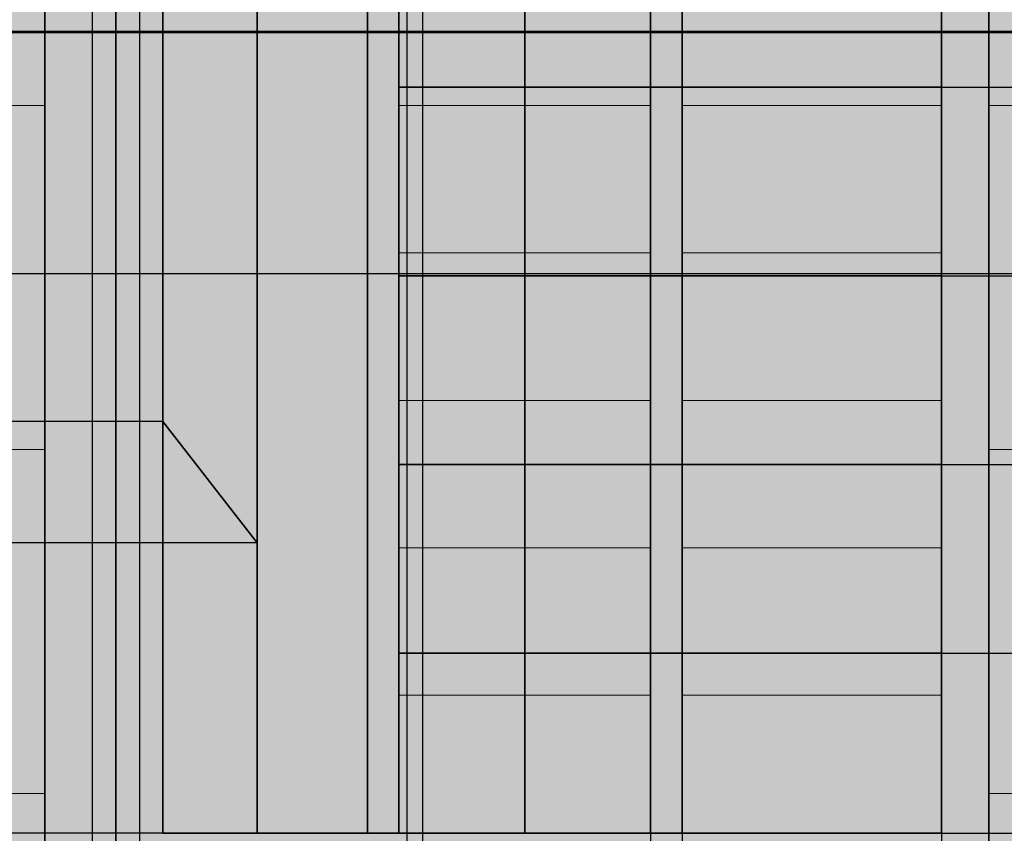
# Model space of a CAD drawing. Units: inches. Extents: x 148 to 1080, y 89 to 707.
# Tile 3 of 12: x 272 to 397, y 170 to 273. Entities that reach past the tile are written whole.
import ezdxf

# ---------------------------------------------------------------- set-up
doc = ezdxf.new("R2010")
doc.units = ezdxf.units.IN
doc.header["$MEASUREMENT"] = 0
for name, color, linetype, lineweight in [('A-ANNO-DIMS', 2, 'Continuous', 18), ('A-ELEV', 7, 'Continuous', 35), ('A-ELEV-PATT', 8, 'Continuous', 13)]:
    doc.layers.add(name, color=color, linetype=linetype, lineweight=lineweight)
doc.styles.get("Standard").update_dxf_attribs({"font": 'arial.ttf'})
doc.dimstyles.get("Standard").update_dxf_attribs({"dimtxt": 6, "dimasz": 0.18, "dimexe": 0.18, "dimexo": 0.0625, "dimgap": 0.09, "dimtad": 0, "dimtih": 1, "dimtoh": 1, "dimdec": 0, "dimzin": 0, "dimdsep": 46, "dimlunit": 3, "dimtxsty": 'Standard', "dimcen": 0.09, "dimadec": 0, "dimazin": 0, "dimtfac": 1, "dimtdec": 0, "dimtofl": 0, "dimtmove": 0, "dimatfit": 3, "dimfxl": 1, "dimtolj": 1, "dimtzin": 0, "dimarcsym": 0})

# ---------------------------------------------------------------- blocks, each defined once
blk = doc.blocks.new('*D28')
at = {"layer": 'A-ANNO-DIMS', "color": 0, "lineweight": -2, "transparency": 16777216}
for p, q in [((274.96, 331.95), (160.42, 331.95)), ((160.6, 331.77), (160.6, 251.1)), ((160.6, 164.13), (160.6, 244.79)), ((274.96, 163.95), (160.42, 163.95))]:
    blk.add_line(p, q, dxfattribs=at)
at = {"layer": 'A-ANNO-DIMS', "color": 0, "transparency": 16777216}
for points in [[(160.57, 331.77), (160.63, 331.77), (160.6, 331.95)], [(160.57, 164.13), (160.63, 164.13), (160.6, 163.95)]]:
    blk.add_solid(points, dxfattribs=at)
at = {"layer": 'Defpoints', "color": 0, "transparency": 16777216}
for p in [(160.6, 331.95), (275.02, 331.95), (275.02, 163.95)]:
    blk.add_point(p, dxfattribs=at)
at = {"layer": 'A-ANNO-DIMS', "color": 0, "transparency": 16777216, "insert": (160.6, 247.95), "char_height": 6, "attachment_point": 5}
blk.add_mtext('\\A1;168', dxfattribs=at)
blk = doc.blocks.new('*D32')
at = {"layer": 'A-ANNO-DIMS', "color": 0, "lineweight": -2, "transparency": 16777216}
for p, q in [((587, 271.77), (160.42, 271.77)), ((160.6, 271.59), (160.6, 213.18)), ((160.6, 148.46), (160.6, 206.87)), ((587, 148.28), (160.42, 148.28))]:
    blk.add_line(p, q, dxfattribs=at)
at = {"layer": 'A-ANNO-DIMS', "color": 0, "transparency": 16777216}
for points in [[(160.57, 271.59), (160.63, 271.59), (160.6, 271.77)], [(160.57, 148.46), (160.63, 148.46), (160.6, 148.28)]]:
    blk.add_solid(points, dxfattribs=at)
at = {"layer": 'Defpoints', "color": 0, "transparency": 16777216}
for p in [(160.6, 271.77), (587.06, 271.77), (587.06, 148.28)]:
    blk.add_point(p, dxfattribs=at)
at = {"layer": 'A-ANNO-DIMS', "color": 0, "transparency": 16777216, "insert": (160.6, 210.03), "char_height": 6, "attachment_point": 5}
blk.add_mtext('\\A1;123.5', dxfattribs=at)
blk = doc.blocks.new('*D34')
at = {"layer": 'A-ANNO-DIMS', "color": 0, "lineweight": -2, "transparency": 16777216}
for p, q in [((574.96, 283.95), (160.42, 283.95)), ((160.6, 283.77), (160.6, 212.1)), ((160.6, 134.13), (160.6, 205.79)), ((574.96, 133.95), (160.42, 133.95))]:
    blk.add_line(p, q, dxfattribs=at)
at = {"layer": 'A-ANNO-DIMS', "color": 0, "transparency": 16777216}
for points in [[(160.57, 283.77), (160.63, 283.77), (160.6, 283.95)], [(160.57, 134.13), (160.63, 134.13), (160.6, 133.95)]]:
    blk.add_solid(points, dxfattribs=at)
at = {"layer": 'Defpoints', "color": 0, "transparency": 16777216}
for p in [(575.02, 283.95), (160.6, 133.95), (575.02, 133.95)]:
    blk.add_point(p, dxfattribs=at)
at = {"layer": 'A-ANNO-DIMS', "color": 0, "transparency": 16777216, "insert": (160.6, 208.95), "char_height": 6, "attachment_point": 5}
blk.add_mtext('\\A1;150', dxfattribs=at)
blk = doc.blocks.new('*D38')
at = {"layer": 'A-ANNO-DIMS', "color": 0, "lineweight": -2, "transparency": 16777216}
for p, q in [((934.89, 271.95), (160.42, 271.95)), ((160.6, 271.77), (160.6, 206.1)), ((160.6, 134.13), (160.6, 199.79)), ((934.89, 133.95), (160.42, 133.95))]:
    blk.add_line(p, q, dxfattribs=at)
at = {"layer": 'A-ANNO-DIMS', "color": 0, "transparency": 16777216}
for points in [[(160.57, 271.77), (160.63, 271.77), (160.6, 271.95)], [(160.57, 134.13), (160.63, 134.13), (160.6, 133.95)]]:
    blk.add_solid(points, dxfattribs=at)
at = {"layer": 'Defpoints', "color": 0, "transparency": 16777216}
for p in [(934.95, 271.95), (160.6, 133.95), (934.95, 133.95)]:
    blk.add_point(p, dxfattribs=at)
at = {"layer": 'A-ANNO-DIMS', "color": 0, "transparency": 16777216, "insert": (160.6, 202.95), "char_height": 6, "attachment_point": 5}
blk.add_mtext('\\A1;138', dxfattribs=at)
blk = doc.blocks.new('*D43')
at = {"layer": 'A-ANNO-DIMS', "color": 0, "lineweight": -2, "transparency": 16777216}
for p, q in [((765.88, 241.1), (160.42, 241.1)), ((160.6, 240.92), (160.6, 190.68)), ((160.6, 134.13), (160.6, 184.37)), ((776.65, 133.95), (160.42, 133.95))]:
    blk.add_line(p, q, dxfattribs=at)
at = {"layer": 'A-ANNO-DIMS', "color": 0, "transparency": 16777216}
for points in [[(160.57, 240.92), (160.63, 240.92), (160.6, 241.1)], [(160.57, 134.13), (160.63, 134.13), (160.6, 133.95)]]:
    blk.add_solid(points, dxfattribs=at)
at = {"layer": 'Defpoints', "color": 0, "transparency": 16777216}
for p in [(765.95, 241.1), (160.6, 133.95), (776.71, 133.95)]:
    blk.add_point(p, dxfattribs=at)
at = {"layer": 'A-ANNO-DIMS', "color": 0, "transparency": 16777216, "insert": (160.6, 187.52), "char_height": 6, "attachment_point": 5}
blk.add_mtext('\\A1;107.15', dxfattribs=at)
blk = doc.blocks.new('*D71')
at = {"layer": 'A-ANNO-DIMS', "color": 0, "lineweight": -2, "transparency": 16777216}
for p, q in [((389.08, 169.95), (1064.5, 169.95)), ((1064.32, 169.95), (1064.32, 170.13)), ((1064.32, 170.13), (1064.5, 170.13)), ((1064.32, 164.13), (1064.32, 169.77)), ((395.08, 163.95), (1064.5, 163.95))]:
    blk.add_line(p, q, dxfattribs=at)
at = {"layer": 'A-ANNO-DIMS', "color": 0, "transparency": 16777216}
for points in [[(1064.29, 169.77), (1064.35, 169.77), (1064.32, 169.95)], [(1064.29, 164.13), (1064.35, 164.13), (1064.32, 163.95)]]:
    blk.add_solid(points, dxfattribs=at)
at = {"layer": 'Defpoints', "color": 0, "transparency": 16777216}
for p in [(389.02, 169.95), (1064.32, 169.95), (395.02, 163.95)]:
    blk.add_point(p, dxfattribs=at)
at = {"layer": 'A-ANNO-DIMS', "color": 0, "transparency": 16777216, "insert": (1072.39, 170.13), "char_height": 6, "attachment_point": 5}
blk.add_mtext('\\A1;6.00', dxfattribs=at)
blk = doc.blocks.new('*D72')
at = {"layer": 'A-ANNO-DIMS', "color": 0, "lineweight": -2, "transparency": 16777216}
for p, q in [((389.08, 192.87), (1064.5, 192.87)), ((1064.32, 192.69), (1064.32, 184.56)), ((1064.32, 170.13), (1064.32, 178.26)), ((389.08, 169.95), (1064.5, 169.95))]:
    blk.add_line(p, q, dxfattribs=at)
at = {"layer": 'A-ANNO-DIMS', "color": 0, "transparency": 16777216}
for points in [[(1064.29, 192.69), (1064.35, 192.69), (1064.32, 192.87)], [(1064.29, 170.13), (1064.35, 170.13), (1064.32, 169.95)]]:
    blk.add_solid(points, dxfattribs=at)
at = {"layer": 'Defpoints', "color": 0, "transparency": 16777216}
for p in [(389.02, 192.87), (1064.32, 192.87), (389.02, 169.95)]:
    blk.add_point(p, dxfattribs=at)
at = {"layer": 'A-ANNO-DIMS', "color": 0, "transparency": 16777216, "insert": (1064.32, 181.41), "char_height": 6, "attachment_point": 5}
blk.add_mtext('\\A1;22.92', dxfattribs=at)
blk = doc.blocks.new('*D73')
at = {"layer": 'A-ANNO-DIMS', "color": 0, "lineweight": -2, "transparency": 16777216}
for p, q in [((389.08, 216.87), (1064.5, 216.87)), ((1064.32, 216.69), (1064.32, 208.02)), ((1064.32, 193.05), (1064.32, 201.72)), ((389.08, 192.87), (1064.5, 192.87))]:
    blk.add_line(p, q, dxfattribs=at)
at = {"layer": 'A-ANNO-DIMS', "color": 0, "transparency": 16777216}
for points in [[(1064.29, 216.69), (1064.35, 216.69), (1064.32, 216.87)], [(1064.29, 193.05), (1064.35, 193.05), (1064.32, 192.87)]]:
    blk.add_solid(points, dxfattribs=at)
at = {"layer": 'Defpoints', "color": 0, "transparency": 16777216}
for p in [(389.02, 216.87), (1064.32, 216.87), (389.02, 192.87)]:
    blk.add_point(p, dxfattribs=at)
at = {"layer": 'A-ANNO-DIMS', "color": 0, "transparency": 16777216, "insert": (1064.32, 204.87), "char_height": 6, "attachment_point": 5}
blk.add_mtext('\\A1;24.00', dxfattribs=at)
blk = doc.blocks.new('*D74')
at = {"layer": 'A-ANNO-DIMS', "color": 0, "lineweight": -2, "transparency": 16777216}
for p, q in [((389.08, 240.87), (1064.5, 240.87)), ((1064.32, 240.69), (1064.32, 232.02)), ((1064.32, 217.05), (1064.32, 225.72)), ((389.08, 216.87), (1064.5, 216.87))]:
    blk.add_line(p, q, dxfattribs=at)
at = {"layer": 'A-ANNO-DIMS', "color": 0, "transparency": 16777216}
for points in [[(1064.29, 240.69), (1064.35, 240.69), (1064.32, 240.87)], [(1064.29, 217.05), (1064.35, 217.05), (1064.32, 216.87)]]:
    blk.add_solid(points, dxfattribs=at)
at = {"layer": 'Defpoints', "color": 0, "transparency": 16777216}
for p in [(389.02, 240.87), (1064.32, 240.87), (389.02, 216.87)]:
    blk.add_point(p, dxfattribs=at)
at = {"layer": 'A-ANNO-DIMS', "color": 0, "transparency": 16777216, "insert": (1064.32, 228.87), "char_height": 6, "attachment_point": 5}
blk.add_mtext('\\A1;24.00', dxfattribs=at)
blk = doc.blocks.new('*D75')
at = {"layer": 'A-ANNO-DIMS', "color": 0, "lineweight": -2, "transparency": 16777216}
for p, q in [((389.08, 264.87), (1064.5, 264.87)), ((1064.32, 264.69), (1064.32, 256.02)), ((1064.32, 241.05), (1064.32, 249.72)), ((389.08, 240.87), (1064.5, 240.87))]:
    blk.add_line(p, q, dxfattribs=at)
at = {"layer": 'A-ANNO-DIMS', "color": 0, "transparency": 16777216}
for points in [[(1064.29, 264.69), (1064.35, 264.69), (1064.32, 264.87)], [(1064.29, 241.05), (1064.35, 241.05), (1064.32, 240.87)]]:
    blk.add_solid(points, dxfattribs=at)
at = {"layer": 'Defpoints', "color": 0, "transparency": 16777216}
for p in [(389.02, 264.87), (1064.32, 264.87), (389.02, 240.87)]:
    blk.add_point(p, dxfattribs=at)
at = {"layer": 'A-ANNO-DIMS', "color": 0, "transparency": 16777216, "insert": (1064.32, 252.87), "char_height": 6, "attachment_point": 5}
blk.add_mtext('\\A1;24.00', dxfattribs=at)
blk = doc.blocks.new('*D76')
at = {"layer": 'A-ANNO-DIMS', "color": 0, "lineweight": -2, "transparency": 16777216}
for p, q in [((389.08, 300.95), (1064.5, 300.95)), ((1064.32, 300.77), (1064.32, 286.06)), ((1064.32, 265.05), (1064.32, 279.75)), ((389.08, 264.87), (1064.5, 264.87))]:
    blk.add_line(p, q, dxfattribs=at)
at = {"layer": 'A-ANNO-DIMS', "color": 0, "transparency": 16777216}
for points in [[(1064.29, 300.77), (1064.35, 300.77), (1064.32, 300.95)], [(1064.29, 265.05), (1064.35, 265.05), (1064.32, 264.87)]]:
    blk.add_solid(points, dxfattribs=at)
at = {"layer": 'Defpoints', "color": 0, "transparency": 16777216}
for p in [(389.02, 300.95), (1064.32, 300.95), (389.02, 264.87)]:
    blk.add_point(p, dxfattribs=at)
at = {"layer": 'A-ANNO-DIMS', "color": 0, "transparency": 16777216, "insert": (1064.32, 282.91), "char_height": 6, "attachment_point": 5}
blk.add_mtext('\\A1;36.08', dxfattribs=at)
blk = doc.blocks.new('*D80')
at = {"layer": 'A-ANNO-DIMS', "color": 0, "lineweight": -2, "transparency": 16777216}
for p, q in [((289.96, 222.32), (160.42, 222.32)), ((160.6, 222.14), (160.6, 199.29)), ((160.6, 170.13), (160.6, 192.98)), ((289.96, 169.95), (160.42, 169.95))]:
    blk.add_line(p, q, dxfattribs=at)
at = {"layer": 'A-ANNO-DIMS', "color": 0, "transparency": 16777216}
for points in [[(160.57, 222.14), (160.63, 222.14), (160.6, 222.32)], [(160.57, 170.13), (160.63, 170.13), (160.6, 169.95)]]:
    blk.add_solid(points, dxfattribs=at)
at = {"layer": 'Defpoints', "color": 0, "transparency": 16777216}
for p in [(160.6, 222.32), (290.02, 222.32), (290.02, 169.95)]:
    blk.add_point(p, dxfattribs=at)
at = {"layer": 'A-ANNO-DIMS', "color": 0, "transparency": 16777216, "insert": (160.6, 196.13), "char_height": 6, "attachment_point": 5}
blk.add_mtext('\\A1;52.37', dxfattribs=at)
blk = doc.blocks.new('*D81')
at = {"layer": 'A-ANNO-DIMS', "color": 0, "lineweight": -2, "transparency": 16777216}
for p, q in [((301.96, 206.89), (160.42, 206.89)), ((160.6, 206.71), (160.6, 191.57)), ((160.6, 170.13), (160.6, 185.26)), ((301.96, 169.95), (160.42, 169.95))]:
    blk.add_line(p, q, dxfattribs=at)
at = {"layer": 'A-ANNO-DIMS', "color": 0, "transparency": 16777216}
for points in [[(160.57, 206.71), (160.63, 206.71), (160.6, 206.89)], [(160.57, 170.13), (160.63, 170.13), (160.6, 169.95)]]:
    blk.add_solid(points, dxfattribs=at)
at = {"layer": 'Defpoints', "color": 0, "transparency": 16777216}
for p in [(160.6, 206.89), (302.02, 206.89), (302.02, 169.95)]:
    blk.add_point(p, dxfattribs=at)
at = {"layer": 'A-ANNO-DIMS', "color": 0, "transparency": 16777216, "insert": (160.6, 188.42), "char_height": 6, "attachment_point": 5}
blk.add_mtext('\\A1;36.944', dxfattribs=at)
blk = doc.blocks.new('*D82')
at = {"layer": 'A-ANNO-DIMS', "color": 0, "lineweight": -2, "transparency": 16777216}
for p, q in [((275.02, 400.88), (275.02, 92.62)), ((281.02, 400.88), (281.02, 92.62)), ((275.2, 92.8), (280.84, 92.8)), ((281.02, 92.8), (281.2, 92.8))]:
    blk.add_line(p, q, dxfattribs=at)
at = {"layer": 'A-ANNO-DIMS', "color": 0, "transparency": 16777216}
for points in [[(275.2, 92.83), (275.2, 92.77), (275.02, 92.8)], [(280.84, 92.83), (280.84, 92.77), (281.02, 92.8)]]:
    blk.add_solid(points, dxfattribs=at)
at = {"layer": 'Defpoints', "color": 0, "transparency": 16777216}
for p in [(275.02, 400.95), (281.02, 400.95), (281.02, 92.8)]:
    blk.add_point(p, dxfattribs=at)
at = {"layer": 'A-ANNO-DIMS', "color": 0, "transparency": 16777216, "insert": (289.09, 92.8), "char_height": 6, "attachment_point": 5}
blk.add_mtext('\\A1;6.00', dxfattribs=at)
blk = doc.blocks.new('*D83')
at = {"layer": 'A-ANNO-DIMS', "color": 0, "lineweight": -2, "transparency": 16777216}
for p, q in [((281.02, 400.88), (281.02, 92.62)), ((287.02, 400.88), (287.02, 92.62)), ((281.2, 92.8), (286.84, 92.8)), ((287.02, 92.8), (287.2, 92.8))]:
    blk.add_line(p, q, dxfattribs=at)
at = {"layer": 'A-ANNO-DIMS', "color": 0, "transparency": 16777216}
for points in [[(281.2, 92.83), (281.2, 92.77), (281.02, 92.8)], [(286.84, 92.83), (286.84, 92.77), (287.02, 92.8)]]:
    blk.add_solid(points, dxfattribs=at)
at = {"layer": 'Defpoints', "color": 0, "transparency": 16777216}
for p in [(281.02, 400.95), (287.02, 400.95), (287.02, 92.8)]:
    blk.add_point(p, dxfattribs=at)
at = {"layer": 'A-ANNO-DIMS', "color": 0, "transparency": 16777216, "insert": (295.09, 92.8), "char_height": 6, "attachment_point": 5}
blk.add_mtext('\\A1;6.00', dxfattribs=at)
blk = doc.blocks.new('*D84')
at = {"layer": 'A-ANNO-DIMS', "color": 0, "lineweight": -2, "transparency": 16777216}
for p, q in [((321.02, 529.88), (321.02, 92.62)), ((287.02, 400.88), (287.02, 92.62)), ((287.2, 92.8), (293.82, 92.8)), ((320.84, 92.8), (314.22, 92.8))]:
    blk.add_line(p, q, dxfattribs=at)
at = {"layer": 'A-ANNO-DIMS', "color": 0, "transparency": 16777216}
for points in [[(287.2, 92.83), (287.2, 92.77), (287.02, 92.8)], [(320.84, 92.83), (320.84, 92.77), (321.02, 92.8)]]:
    blk.add_solid(points, dxfattribs=at)
at = {"layer": 'Defpoints', "color": 0, "transparency": 16777216}
for p in [(321.02, 529.95), (287.02, 400.95), (321.02, 92.8)]:
    blk.add_point(p, dxfattribs=at)
at = {"layer": 'A-ANNO-DIMS', "color": 0, "transparency": 16777216, "insert": (304.02, 92.8), "char_height": 6, "attachment_point": 5}
blk.add_mtext('\\A1;34.00', dxfattribs=at)
blk = doc.blocks.new('*D85')
at = {"layer": 'A-ANNO-DIMS', "color": 0, "lineweight": -2, "transparency": 16777216}
for p, q in [((321.02, 529.88), (321.02, 92.62)), ((323.02, 400.88), (323.02, 92.62)), ((321.2, 92.8), (322.84, 92.8)), ((323.02, 92.8), (323.2, 92.8))]:
    blk.add_line(p, q, dxfattribs=at)
at = {"layer": 'A-ANNO-DIMS', "color": 0, "transparency": 16777216}
for points in [[(321.2, 92.83), (321.2, 92.77), (321.02, 92.8)], [(322.84, 92.83), (322.84, 92.77), (323.02, 92.8)]]:
    blk.add_solid(points, dxfattribs=at)
at = {"layer": 'Defpoints', "color": 0, "transparency": 16777216}
for p in [(321.02, 529.95), (323.02, 400.95), (323.02, 92.8)]:
    blk.add_point(p, dxfattribs=at)
at = {"layer": 'A-ANNO-DIMS', "color": 0, "transparency": 16777216, "insert": (331.12, 92.8), "char_height": 6, "attachment_point": 5}
blk.add_mtext('\\A1;2.00', dxfattribs=at)
blk = doc.blocks.new('*D86')
at = {"layer": 'A-ANNO-DIMS', "color": 0, "lineweight": -2, "transparency": 16777216}
for p, q in [((323.02, 400.88), (323.02, 92.62)), ((352.02, 400.88), (352.02, 92.62)), ((323.2, 92.8), (327.27, 92.8)), ((351.84, 92.8), (347.77, 92.8))]:
    blk.add_line(p, q, dxfattribs=at)
at = {"layer": 'A-ANNO-DIMS', "color": 0, "transparency": 16777216}
for points in [[(323.2, 92.83), (323.2, 92.77), (323.02, 92.8)], [(351.84, 92.83), (351.84, 92.77), (352.02, 92.8)]]:
    blk.add_solid(points, dxfattribs=at)
at = {"layer": 'Defpoints', "color": 0, "transparency": 16777216}
for p in [(323.02, 400.95), (352.02, 400.95), (352.02, 92.8)]:
    blk.add_point(p, dxfattribs=at)
at = {"layer": 'A-ANNO-DIMS', "color": 0, "transparency": 16777216, "insert": (337.52, 92.8), "char_height": 6, "attachment_point": 5}
blk.add_mtext('\\A1;29.00', dxfattribs=at)
blk = doc.blocks.new('*D87')
at = {"layer": 'A-ANNO-DIMS', "color": 0, "lineweight": -2, "transparency": 16777216}
for p, q in [((352.02, 400.88), (352.02, 92.62)), ((356.02, 400.88), (356.02, 92.62)), ((352.2, 92.8), (355.84, 92.8)), ((356.02, 92.8), (356.2, 92.8))]:
    blk.add_line(p, q, dxfattribs=at)
at = {"layer": 'A-ANNO-DIMS', "color": 0, "transparency": 16777216}
for points in [[(352.2, 92.83), (352.2, 92.77), (352.02, 92.8)], [(355.84, 92.83), (355.84, 92.77), (356.02, 92.8)]]:
    blk.add_solid(points, dxfattribs=at)
at = {"layer": 'Defpoints', "color": 0, "transparency": 16777216}
for p in [(352.02, 400.95), (356.02, 400.95), (356.02, 92.8)]:
    blk.add_point(p, dxfattribs=at)
at = {"layer": 'A-ANNO-DIMS', "color": 0, "transparency": 16777216, "insert": (364.19, 92.8), "char_height": 6, "attachment_point": 5}
blk.add_mtext('\\A1;4.00', dxfattribs=at)
blk = doc.blocks.new('*D88')
at = {"layer": 'A-ANNO-DIMS', "color": 0, "lineweight": -2, "transparency": 16777216}
for p, q in [((356.02, 400.88), (356.02, 92.62)), ((389.02, 400.88), (389.02, 92.62)), ((356.2, 92.8), (362.32, 92.8)), ((388.84, 92.8), (382.72, 92.8))]:
    blk.add_line(p, q, dxfattribs=at)
at = {"layer": 'A-ANNO-DIMS', "color": 0, "transparency": 16777216}
for points in [[(356.2, 92.83), (356.2, 92.77), (356.02, 92.8)], [(388.84, 92.83), (388.84, 92.77), (389.02, 92.8)]]:
    blk.add_solid(points, dxfattribs=at)
at = {"layer": 'Defpoints', "color": 0, "transparency": 16777216}
for p in [(356.02, 400.95), (389.02, 400.95), (389.02, 92.8)]:
    blk.add_point(p, dxfattribs=at)
at = {"layer": 'A-ANNO-DIMS', "color": 0, "transparency": 16777216, "insert": (372.52, 92.8), "char_height": 6, "attachment_point": 5}
blk.add_mtext('\\A1;33.00', dxfattribs=at)
blk = doc.blocks.new('*D89')
at = {"layer": 'A-ANNO-DIMS', "color": 0, "lineweight": -2, "transparency": 16777216}
for p, q in [((389.02, 400.88), (389.02, 92.62)), ((395.02, 400.88), (395.02, 92.62)), ((389.2, 92.8), (394.84, 92.8)), ((395.02, 92.8), (395.2, 92.8))]:
    blk.add_line(p, q, dxfattribs=at)
at = {"layer": 'A-ANNO-DIMS', "color": 0, "transparency": 16777216}
for points in [[(389.2, 92.83), (389.2, 92.77), (389.02, 92.8)], [(394.84, 92.83), (394.84, 92.77), (395.02, 92.8)]]:
    blk.add_solid(points, dxfattribs=at)
at = {"layer": 'Defpoints', "color": 0, "transparency": 16777216}
for p in [(389.02, 400.95), (395.02, 400.95), (395.02, 92.8)]:
    blk.add_point(p, dxfattribs=at)
at = {"layer": 'A-ANNO-DIMS', "color": 0, "transparency": 16777216, "insert": (403.09, 92.8), "char_height": 6, "attachment_point": 5}
blk.add_mtext('\\A1;6.00', dxfattribs=at)
blk = doc.blocks.new('*D102')
at = {"layer": 'A-ANNO-DIMS', "color": 0, "lineweight": -2, "transparency": 16777216}
for p, q in [((742.96, 271.95), (160.42, 271.95)), ((160.6, 271.77), (160.6, 259.68)), ((160.6, 241.28), (160.6, 253.37)), ((765.88, 241.1), (160.42, 241.1))]:
    blk.add_line(p, q, dxfattribs=at)
at = {"layer": 'A-ANNO-DIMS', "color": 0, "transparency": 16777216}
for points in [[(160.57, 271.77), (160.63, 271.77), (160.6, 271.95)], [(160.57, 241.28), (160.63, 241.28), (160.6, 241.1)]]:
    blk.add_solid(points, dxfattribs=at)
at = {"layer": 'Defpoints', "color": 0, "transparency": 16777216}
for p in [(160.6, 271.95), (743.02, 271.95), (765.95, 241.1)]:
    blk.add_point(p, dxfattribs=at)
at = {"layer": 'A-ANNO-DIMS', "color": 0, "transparency": 16777216, "insert": (160.6, 256.52), "char_height": 6, "attachment_point": 5}
blk.add_mtext('\\A1;30.85', dxfattribs=at)

msp = doc.modelspace()

# ---------------------------------------------------------------- hatches: boundary and pattern name
at = {"layer": 'A-ELEV-PATT'}
h = msp.add_hatch(color=256, dxfattribs=at)
h.dxf.hatch_style = 1
h.paths.add_polyline_path([(395.0199, 349.9474), (275.0199, 349.9474), (275.0199, 331.9474), (395.0199, 331.9474)])
h.paths.add_polyline_path([(284.0199, 331.9474), (275.0199, 331.9474), (275.0199, 163.9474), (284.0199, 163.9474)])
h.paths.add_polyline_path([(395.0199, 601.9474), (251.0199, 601.9474), (251.0199, 589.9474), (395.0199, 589.9474)])
h = msp.add_hatch(color=256, dxfattribs=at)
h.dxf.hatch_style = 1
h.paths.add_polyline_path([(302.0199, 206.8913), (290.0199, 222.3199), (290.0199, 169.9474), (302.0199, 169.9474)])
h.paths.add_polyline_path([(302.7628, 473.6405), (287.0199, 497.1899), (287.0199, 400.9474), (302.7628, 400.9474)])
h = msp.add_hatch(color=256, dxfattribs=at)
h.dxf.hatch_style = 1
h.paths.add_polyline_path([(527.0199, 349.9474), (395.0199, 349.9474), (395.0199, 271.2774), (527.0199, 272.3839)])
h.paths.add_polyline_path([(275.0199, 349.9474), (251.0199, 349.9474), (251.0199, 270.0704), (275.0199, 270.2716)])
h.paths.add_polyline_path([(743.0199, 337.9474), (734.0628, 337.9474), (719.0199, 326.3632), (719.0199, 277.9474), (743.0199, 277.9474)])
h.paths.add_polyline_path([(743.0199, 277.9474), (719.0199, 277.9474), (719.0199, 133.9474), (743.0199, 133.9474)])
h.paths.add_polyline_path([(734.0628, 337.9474), (719.0199, 337.9474), (719.0199, 326.3632)])
h = msp.add_hatch(dxfattribs=at)
h.set_pattern_fill('ANSI37', color=256, scale=350, angle=135)
h.paths.add_polyline_path([(527.0199, 349.9474), (395.0199, 349.9474), (395.0199, 163.9474), (275.0199, 163.9474), (275.0199, 349.9474), (251.0199, 349.9474), (251.0199, 133.9474), (527.0199, 133.9474)])
h = msp.add_hatch(color=256, dxfattribs=at)
h.dxf.hatch_style = 1
h.paths.add_polyline_path([(527.0199, 272.3839), (395.0199, 271.2774), (395.0199, 163.9474), (275.0199, 163.9474), (275.0199, 270.2716), (251.0199, 270.0704), (251.0199, 133.9474), (527.0199, 133.9474)])
h.paths.add_polyline_path([(1006.9492, 337.9474), (946.9492, 337.9474), (946.9492, 277.9474), (1006.9492, 277.9474)])
h.paths.add_polyline_path([(1006.9492, 277.9474), (946.9492, 277.9474), (946.9492, 133.9474), (1006.9492, 133.9474)])
h.paths.add_polyline_path([(946.9492, 337.9474), (743.0199, 337.9474), (743.0199, 277.9474), (946.9492, 277.9474)])
h = msp.add_hatch(color=256, dxfattribs=at)
h.dxf.hatch_style = 1
h.paths.add_polyline_path([(290.0199, 331.9474), (284.0199, 331.9474), (284.0199, 163.9474), (395.0199, 163.9474), (395.0199, 331.9474), (290.0199, 331.9474), (290.0199, 325.9474), (352.0199, 325.9474), (352.0199, 304.9474), (356.0199, 304.9474), (356.0199, 325.9474), (389.0199, 325.9474), (389.0199, 169.9474), (290.0199, 169.9474)])
h.paths.add_polyline_path([(356.0199, 300.9474), (352.0199, 300.9474), (352.0199, 169.9474), (356.0199, 169.9474)], flags=17)
h.paths.add_polyline_path([(356.0199, 304.9474), (352.0199, 304.9474), (352.0199, 300.9474), (356.0199, 300.9474)], flags=17)
h = msp.add_hatch(color=256, dxfattribs=at)
h.dxf.hatch_style = 1
h.paths.add_polyline_path([(389.0199, 300.9474), (356.0199, 300.9474), (356.0199, 264.8696), (389.0199, 264.8696)])
h.paths.add_polyline_path([(389.0199, 325.9474), (356.0199, 325.9474), (356.0199, 304.9474), (389.0199, 304.9474)])
h.paths.add_polyline_path([(352.0199, 325.9474), (302.0199, 325.9474), (316.0199, 304.9474), (352.0199, 304.9474)])
h.paths.add_polyline_path([(316.0199, 304.9474), (302.0199, 325.9474), (302.0199, 169.9474), (316.0199, 169.9474)])
h.paths.add_polyline_path([(302.0199, 325.9474), (290.0199, 325.9474), (290.0199, 222.3199), (302.0199, 206.8913)])
h.paths.add_polyline_path([(320.0199, 300.9474), (352.0199, 300.9474), (352.0199, 304.9474), (316.0199, 304.9474), (316.0199, 169.9474), (320.0199, 169.9474)])
h.paths.add_polyline_path([(336.0199, 300.9474), (320.0199, 300.9474), (320.0199, 264.8696), (336.0199, 264.8696)], flags=17)
h.paths.add_polyline_path([(352.0199, 300.9474), (336.0199, 300.9474), (336.0199, 264.8696), (352.0199, 264.8696)])
h.paths.add_polyline_path([(389.0199, 304.9474), (356.0199, 304.9474), (356.0199, 300.9474), (389.0199, 300.9474)])
h.paths.add_polyline_path([(389.0199, 192.8696), (356.0199, 192.8696), (356.0199, 169.9474), (389.0199, 169.9474)])
h.paths.add_polyline_path([(389.0199, 216.8696), (356.0199, 216.8696), (356.0199, 192.8696), (389.0199, 192.8696)])
h.paths.add_polyline_path([(389.0199, 240.8696), (356.0199, 240.8696), (356.0199, 216.8696), (389.0199, 216.8696)])
h.paths.add_polyline_path([(389.0199, 264.8696), (356.0199, 264.8696), (356.0199, 240.8696), (389.0199, 240.8696)])
h.paths.add_polyline_path([(352.0199, 264.8696), (336.0199, 264.8696), (336.0199, 240.8696), (352.0199, 240.8696)])
h.paths.add_polyline_path([(336.0199, 264.8696), (320.0199, 264.8696), (320.0199, 240.8696), (336.0199, 240.8696)], flags=17)
h.paths.add_polyline_path([(336.0199, 240.8696), (320.0199, 240.8696), (320.0199, 216.8696), (336.0199, 216.8696)], flags=17)
h.paths.add_polyline_path([(352.0199, 240.8696), (336.0199, 240.8696), (336.0199, 216.8696), (352.0199, 216.8696)])
h.paths.add_polyline_path([(352.0199, 216.8696), (336.0199, 216.8696), (336.0199, 192.8696), (352.0199, 192.8696)])
h.paths.add_polyline_path([(336.0199, 216.8696), (320.0199, 216.8696), (320.0199, 192.8696), (336.0199, 192.8696)], flags=17)
h.paths.add_polyline_path([(336.0199, 192.8696), (320.0199, 192.8696), (320.0199, 169.9474), (336.0199, 169.9474)], flags=17)
h.paths.add_polyline_path([(352.0199, 192.8696), (336.0199, 192.8696), (336.0199, 169.9474), (352.0199, 169.9474)])
h = msp.add_hatch(dxfattribs=at)
h.set_pattern_fill('ANSI31', color=256, scale=150, angle=135)
h.paths.add_polyline_path([(389.0199, 192.8696), (356.0199, 192.8696), (356.0199, 169.9474), (389.0199, 169.9474)])
h.paths.add_polyline_path([(389.0199, 240.8696), (356.0199, 240.8696), (356.0199, 216.8696), (389.0199, 216.8696)])
h.paths.add_polyline_path([(389.0199, 216.8696), (356.0199, 216.8696), (356.0199, 192.8696), (389.0199, 192.8696)])
h.paths.add_polyline_path([(389.0199, 264.8696), (356.0199, 264.8696), (356.0199, 240.8696), (389.0199, 240.8696)])
h.paths.add_polyline_path([(389.0199, 300.9474), (356.0199, 300.9474), (356.0199, 264.8696), (389.0199, 264.8696)])
h.paths.add_polyline_path([(352.0199, 300.9474), (336.0199, 300.9474), (336.0199, 264.8696), (352.0199, 264.8696)])
h.paths.add_polyline_path([(336.0199, 300.9474), (320.0199, 300.9474), (320.0199, 264.8696), (336.0199, 264.8696)])
h.paths.add_polyline_path([(336.0199, 264.8696), (320.0199, 264.8696), (320.0199, 240.8696), (336.0199, 240.8696)])
h.paths.add_polyline_path([(352.0199, 264.8696), (336.0199, 264.8696), (336.0199, 240.8696), (352.0199, 240.8696)])
h.paths.add_polyline_path([(336.0199, 240.8696), (320.0199, 240.8696), (320.0199, 216.8696), (336.0199, 216.8696)])
h.paths.add_polyline_path([(352.0199, 240.8696), (336.0199, 240.8696), (336.0199, 216.8696), (352.0199, 216.8696)])
h.paths.add_polyline_path([(336.0199, 216.8696), (320.0199, 216.8696), (320.0199, 192.8696), (336.0199, 192.8696)])
h.paths.add_polyline_path([(352.0199, 216.8696), (336.0199, 216.8696), (336.0199, 192.8696), (352.0199, 192.8696)])
h.paths.add_polyline_path([(336.0199, 192.8696), (320.0199, 192.8696), (320.0199, 169.9474), (336.0199, 169.9474)])
h.paths.add_polyline_path([(352.0199, 192.8696), (336.0199, 192.8696), (336.0199, 169.9474), (352.0199, 169.9474)])

# ---------------------------------------------------------------- linework, layer by layer
at = {"layer": 'A-ELEV'}
for p, q in [((275.0199, 163.9474), (275.0199, 349.9474)), ((395.0199, 163.9474), (395.0199, 349.9474)), ((284.0199, 163.9474), (284.0199, 331.9474)), ((290.0199, 169.9474), (290.0199, 331.9474)), ((302.0199, 169.9474), (302.0199, 325.9474)), ((352.0199, 169.9474), (352.0199, 325.9474)), ((356.0199, 169.9474), (356.0199, 325.9474)), ((389.0199, 169.9474), (389.0199, 325.9474)), ((316.0199, 169.9474), (316.0199, 304.9474)), ((320.0199, 169.9474), (320.0199, 300.9474)), ((336.0199, 169.9474), (336.0199, 300.9474)), ((320.0199, 264.8696), (389.0199, 264.8696)), ((320.0199, 240.8696), (389.0199, 240.8696)), ((290.0199, 222.3199), (302.0199, 206.8913)), ((320.0199, 216.8696), (389.0199, 216.8696)), ((320.0199, 192.8696), (389.0199, 192.8696)), ((290.0199, 169.9474), (389.0199, 169.9474)), ((293.0199, 169.9474), (347.0199, 169.9474))]:
    msp.add_line(p, q, dxfattribs=at)

# ---------------------------------------------------------------- dimensions: what is measured, and where the dimension line sits
at = {"layer": 'A-ANNO-DIMS'}
for base, p1, p2, picture, middle in [((321.0199, 92.7974), (287.0199, 400.9474), (321.0199, 529.9474), '*D84', (304.0199, 92.7974)), ((323.0199, 92.7974), (321.0199, 529.9474), (323.0199, 400.9474), '*D85', (331.1234, 92.7974)), ((281.0199, 92.7974), (275.0199, 400.9474), (281.0199, 400.9474), '*D82', (289.0886, 92.7974)), ((287.0199, 92.7974), (281.0199, 400.9474), (287.0199, 400.9474), '*D83', (295.0886, 92.7974)), ((352.0199, 92.7974), (323.0199, 400.9474), (352.0199, 400.9474), '*D86', (337.5199, 92.7974)), ((356.0199, 92.7974), (352.0199, 400.9474), (356.0199, 400.9474), '*D87', (364.193, 92.7974)), ((389.0199, 92.7974), (356.0199, 400.9474), (389.0199, 400.9474), '*D88', (372.5199, 92.7974)), ((395.0199, 92.7974), (389.0199, 400.9474), (395.0199, 400.9474), '*D89', (403.0886, 92.7974))]:
    dim = msp.add_linear_dim(base=base, p1=p1, p2=p2, dimstyle='Standard', override={"dimdec": 2, "dimlfac": 1, "dimrnd": 0, "dimzin": 0, "dimdsep": 46, "dimlunit": 2}, dxfattribs=at)
    dim.commit()
    dim.dimension.update_dxf_attribs({"geometry": picture, "text_midpoint": middle})
for base, p1, p2, override, picture, middle in [((160.5992, 331.9474), (275.0199, 163.9474), (275.0199, 331.9474), {"dimdec": 0, "dimlfac": 1, "dimrnd": 0, "dimzin": 0, "dimdsep": 46, "dimlunit": 2}, '*D28', (160.5992, 247.9474)), ((1064.325, 300.9474), (389.0199, 264.8696), (389.0199, 300.9474), {"dimdec": 2, "dimlfac": 1, "dimrnd": 0, "dimzin": 0, "dimdsep": 46, "dimlunit": 2}, '*D76', (1064.325, 282.9085)), ((160.5992, 133.9474), (575.0199, 283.9474), (575.0199, 133.9474), {"dimdec": 0, "dimlfac": 1, "dimrnd": 0, "dimzin": 0, "dimdsep": 46, "dimlunit": 2}, '*D34', (160.5992, 208.9474)), ((160.5992, 271.9474), (765.9474, 241.0996), (743.0199, 271.9474), {"dimdec": 2, "dimlfac": 1, "dimrnd": 0, "dimzin": 0, "dimdsep": 46, "dimlunit": 2}, '*D102', (160.5992, 256.5235)), ((160.5992, 271.7747), (587.0631, 148.2809), (587.0631, 271.7747), {"dimdec": 1, "dimlfac": 1, "dimrnd": 0, "dimzin": 0, "dimdsep": 46, "dimlunit": 2}, '*D32', (160.5992, 210.0278)), ((160.5992, 133.9474), (934.9492, 271.9474), (934.9492, 133.9474), {"dimdec": 0, "dimlfac": 1, "dimrnd": 0, "dimzin": 0, "dimdsep": 46, "dimlunit": 2}, '*D38', (160.5992, 202.9474)), ((1064.325, 264.8696), (389.0199, 240.8696), (389.0199, 264.8696), {"dimdec": 2, "dimlfac": 1, "dimrnd": 0, "dimzin": 0, "dimdsep": 46, "dimlunit": 2}, '*D75', (1064.325, 252.8696)), ((160.5992, 133.9474), (765.9474, 241.0996), (776.713, 133.9474), {"dimdec": 2, "dimlfac": 1, "dimrnd": 0, "dimzin": 0, "dimdsep": 46, "dimlunit": 2}, '*D43', (160.5992, 187.5235)), ((1064.325, 240.8696), (389.0199, 216.8696), (389.0199, 240.8696), {"dimdec": 2, "dimlfac": 1, "dimrnd": 0, "dimzin": 0, "dimdsep": 46, "dimlunit": 2}, '*D74', (1064.325, 228.8696)), ((160.5992, 222.3199), (290.0199, 169.9474), (290.0199, 222.3199), {"dimdec": 2, "dimlfac": 1, "dimrnd": 0, "dimzin": 0, "dimdsep": 46, "dimlunit": 2}, '*D80', (160.5992, 196.1336)), ((1064.325, 216.8696), (389.0199, 192.8696), (389.0199, 216.8696), {"dimdec": 2, "dimlfac": 1, "dimrnd": 0, "dimzin": 0, "dimdsep": 46, "dimlunit": 2}, '*D73', (1064.325, 204.8696)), ((160.5992, 206.8913), (302.0199, 169.9474), (302.0199, 206.8913), {"dimdec": 3, "dimlfac": 1, "dimrnd": 0, "dimzin": 0, "dimdsep": 46, "dimlunit": 2}, '*D81', (160.5992, 188.4194)), ((1064.325, 192.8696), (389.0199, 169.9474), (389.0199, 192.8696), {"dimdec": 2, "dimlfac": 1, "dimrnd": 0, "dimzin": 0, "dimdsep": 46, "dimlunit": 2}, '*D72', (1064.325, 181.4085)), ((1064.325, 169.9474), (395.0199, 163.9474), (389.0199, 169.9474), {"dimdec": 2, "dimlfac": 1, "dimrnd": 0, "dimzin": 0, "dimdsep": 46, "dimlunit": 2}, '*D71', (1072.3937, 170.1274))]:
    dim = msp.add_linear_dim(base=base, p1=p1, p2=p2, angle=90, dimstyle='Standard', override=override, dxfattribs=at)
    dim.commit()
    dim.dimension.update_dxf_attribs({"geometry": picture, "text_midpoint": middle})

doc.saveas('drawing.dxf')
